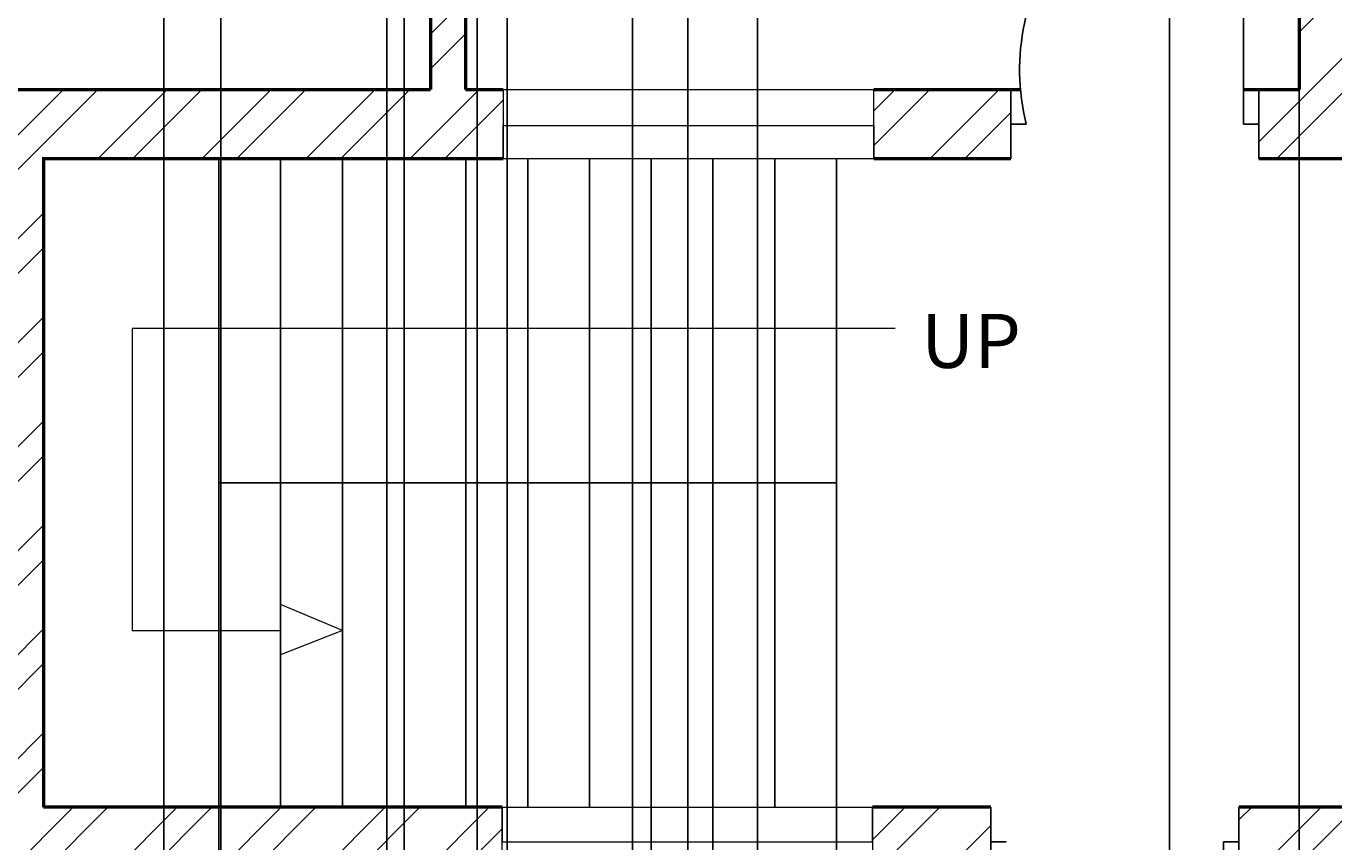
# Model space of a CAD drawing. Units: inches. Extents: x 1980 to 2738, y 1471 to 2568.
# Tile 10 of 22: x 2194 to 2363, y 2007 to 2112. Entities that reach past the tile are written whole.
import ezdxf

# ---------------------------------------------------------------- set-up
doc = ezdxf.new("R2010")
doc.units = ezdxf.units.IN
for name, color, linetype, lineweight in [('A-ANNO-DIMS', 2, 'Continuous', 18), ('A-ANNO-SYMB', 60, 'Continuous', 18), ('A-ANNO-TEXT', 7, 'Continuous', 18), ('A-DOOR', 31, 'Continuous', 25), ('A-FLOR-STRS', 60, 'Continuous', 25), ('A-GLAZ', 141, 'Continuous', 18), ('A-WALL', 7, 'Continuous', 50)]:
    doc.layers.add(name, color=color, linetype=linetype, lineweight=lineweight)
doc.layers.add('A-WALL-PATT', color=9, linetype='Continuous', lineweight=13, true_color=0xd19cc7)
doc.styles.get("Standard").update_dxf_attribs({"font": 'arial.ttf'})
doc.dimstyles.get("Standard").update_dxf_attribs({"dimtxt": 0.18, "dimasz": 0.18, "dimexe": 0.18, "dimexo": 0.0625, "dimgap": 0.09, "dimtad": 0, "dimtih": 1, "dimtoh": 1, "dimdec": 4, "dimzin": 0, "dimdsep": 46, "dimtxsty": 'Standard', "dimcen": 0.09, "dimadec": 0, "dimazin": 0, "dimtfac": 1, "dimtdec": 4, "dimtofl": 0, "dimtmove": 0, "dimatfit": 3, "dimfxl": 1, "dimtolj": 1, "dimtzin": 0, "dimarcsym": 0})

# ---------------------------------------------------------------- blocks, each defined once
blk = doc.blocks.new('WIN-48IN-WALL')
for p, q in [((0, 4.5), (0, 9)), ((0, 9), (0, 0)), ((48, 9), (0, 9)), ((48, 0), (48, 9)), ((48, 9), (48, 4.5)), ((48, 4.5), (0, 4.5)), ((0, 0), (48, 0))]:
    blk.add_line(p, q)
blk = doc.blocks.new('*D40')
at = {"layer": 'A-ANNO-DIMS', "color": 0, "lineweight": -2, "transparency": 16777216}
for p, q in [((2218.65, 2053.14), (2218.65, 1533.71)), ((2298.65, 2053.14), (2298.65, 1533.71)), ((2218.83, 1533.89), (2258.43, 1533.89)), ((2298.47, 1533.89), (2258.87, 1533.89))]:
    blk.add_line(p, q, dxfattribs=at)
at = {"layer": 'A-ANNO-DIMS', "color": 0, "transparency": 16777216}
for points in [[(2218.83, 1533.92), (2218.83, 1533.86), (2218.65, 1533.89)], [(2298.47, 1533.92), (2298.47, 1533.86), (2298.65, 1533.89)]]:
    blk.add_solid(points, dxfattribs=at)
at = {"layer": 'Defpoints', "color": 0, "transparency": 16777216}
for p in [(2218.65, 2053.21), (2298.65, 2053.21), (2298.65, 1533.89)]:
    blk.add_point(p, dxfattribs=at)
at = {"layer": 'A-ANNO-DIMS', "color": 0, "transparency": 16777216, "insert": (2258.65, 1533.89), "char_height": 0.18, "attachment_point": 5}
blk.add_mtext('\\A1;80', dxfattribs=at)
blk = doc.blocks.new('*D41')
at = {"layer": 'A-ANNO-DIMS', "color": 0, "lineweight": -2, "transparency": 16777216}
for p, q in [((2298.65, 2095.14), (2298.65, 1533.71)), ((2515.4, 2095.14), (2515.4, 1533.71)), ((2298.83, 1533.89), (2406.56, 1533.89)), ((2515.22, 1533.89), (2407.49, 1533.89))]:
    blk.add_line(p, q, dxfattribs=at)
at = {"layer": 'A-ANNO-DIMS', "color": 0, "transparency": 16777216}
for points in [[(2298.83, 1533.92), (2298.83, 1533.86), (2298.65, 1533.89)], [(2515.22, 1533.92), (2515.22, 1533.86), (2515.4, 1533.89)]]:
    blk.add_solid(points, dxfattribs=at)
at = {"layer": 'Defpoints', "color": 0, "transparency": 16777216}
for p in [(2298.65, 2095.21), (2515.4, 2095.21), (2515.4, 1533.89)]:
    blk.add_point(p, dxfattribs=at)
at = {"layer": 'A-ANNO-DIMS', "color": 0, "transparency": 16777216, "insert": (2407.03, 1533.89), "char_height": 0.18, "attachment_point": 5}
blk.add_mtext('\\A1;216.75', dxfattribs=at)
blk = doc.blocks.new('*D44')
at = {"layer": 'A-ANNO-DIMS', "color": 0, "lineweight": -2, "transparency": 16777216}
for p, q in [((2218.88, 1694.77), (2218.88, 2507.54)), ((2219.06, 2507.36), (2229.18, 2507.36)), ((2240.22, 2507.36), (2230.11, 2507.36)), ((2240.4, 1694.77), (2240.4, 2507.54))]:
    blk.add_line(p, q, dxfattribs=at)
at = {"layer": 'A-ANNO-DIMS', "color": 0, "transparency": 16777216}
for points in [[(2219.06, 2507.39), (2219.06, 2507.33), (2218.88, 2507.36)], [(2240.22, 2507.39), (2240.22, 2507.33), (2240.4, 2507.36)]]:
    blk.add_solid(points, dxfattribs=at)
at = {"layer": 'Defpoints', "color": 0, "transparency": 16777216}
for p in [(2240.4, 2507.36), (2218.88, 1694.71), (2240.4, 1694.71)]:
    blk.add_point(p, dxfattribs=at)
at = {"layer": 'A-ANNO-DIMS', "color": 0, "transparency": 16777216, "insert": (2229.64, 2507.36), "char_height": 0.18, "attachment_point": 5}
blk.add_mtext('\\A1;21.525', dxfattribs=at)
blk = doc.blocks.new('*D45')
at = {"layer": 'A-ANNO-DIMS', "color": 0, "lineweight": -2, "transparency": 16777216}
for p, q in [((2255.99, 1694.77), (2255.99, 2507.54)), ((2256.17, 2507.36), (2267.22, 2507.36)), ((2279.21, 2507.36), (2268.15, 2507.36)), ((2279.39, 1694.77), (2279.39, 2507.54))]:
    blk.add_line(p, q, dxfattribs=at)
at = {"layer": 'A-ANNO-DIMS', "color": 0, "transparency": 16777216}
for points in [[(2256.17, 2507.39), (2256.17, 2507.33), (2255.99, 2507.36)], [(2279.21, 2507.39), (2279.21, 2507.33), (2279.39, 2507.36)]]:
    blk.add_solid(points, dxfattribs=at)
at = {"layer": 'Defpoints', "color": 0, "transparency": 16777216}
for p in [(2279.39, 2507.36), (2255.99, 1694.71), (2279.39, 1694.71)]:
    blk.add_point(p, dxfattribs=at)
at = {"layer": 'A-ANNO-DIMS', "color": 0, "transparency": 16777216, "insert": (2267.69, 2507.36), "char_height": 0.18, "attachment_point": 5}
blk.add_mtext('\\A1;23.407', dxfattribs=at)
blk = doc.blocks.new('*D46')
at = {"layer": 'A-ANNO-DIMS', "color": 0, "lineweight": -2, "transparency": 16777216}
for p, q in [((2211.52, 1814.77), (2211.52, 2507.54)), ((2211.7, 2507.36), (2226.69, 2507.36)), ((2242.46, 2507.36), (2227.48, 2507.36)), ((2242.64, 1814.77), (2242.64, 2507.54))]:
    blk.add_line(p, q, dxfattribs=at)
at = {"layer": 'A-ANNO-DIMS', "color": 0, "transparency": 16777216}
for points in [[(2211.7, 2507.39), (2211.7, 2507.33), (2211.52, 2507.36)], [(2242.46, 2507.39), (2242.46, 2507.33), (2242.64, 2507.36)]]:
    blk.add_solid(points, dxfattribs=at)
at = {"layer": 'Defpoints', "color": 0, "transparency": 16777216}
for p in [(2242.64, 2507.36), (2211.52, 1814.71), (2242.64, 1814.71)]:
    blk.add_point(p, dxfattribs=at)
at = {"layer": 'A-ANNO-DIMS', "color": 0, "transparency": 16777216, "insert": (2227.08, 2507.36), "char_height": 0.18, "attachment_point": 5}
blk.add_mtext('\\A1;31.12', dxfattribs=at)
blk = doc.blocks.new('*D50')
at = {"layer": 'A-ANNO-DIMS', "color": 0, "lineweight": -2, "transparency": 16777216}
for p, q in [((2288.43, 1708.09), (2288.43, 2507.54)), ((2288.61, 2507.36), (2314.71, 2507.36)), ((2341.6, 2507.36), (2315.5, 2507.36)), ((2341.78, 1708.09), (2341.78, 2507.54))]:
    blk.add_line(p, q, dxfattribs=at)
at = {"layer": 'A-ANNO-DIMS', "color": 0, "transparency": 16777216}
for points in [[(2288.61, 2507.39), (2288.61, 2507.33), (2288.43, 2507.36)], [(2341.6, 2507.39), (2341.6, 2507.33), (2341.78, 2507.36)]]:
    blk.add_solid(points, dxfattribs=at)
at = {"layer": 'Defpoints', "color": 0, "transparency": 16777216}
for p in [(2341.78, 2507.36), (2288.43, 1708.03), (2341.78, 1708.03)]:
    blk.add_point(p, dxfattribs=at)
at = {"layer": 'A-ANNO-DIMS', "color": 0, "transparency": 16777216, "insert": (2315.11, 2507.36), "char_height": 0.18, "attachment_point": 5}
blk.add_mtext('\\A1;53.34', dxfattribs=at)
blk = doc.blocks.new('*D51')
at = {"layer": 'A-ANNO-DIMS', "color": 0, "lineweight": -2, "transparency": 16777216}
for p, q in [((2341.78, 1708.09), (2341.78, 2507.54)), ((2341.96, 2507.36), (2349.72, 2507.36)), ((2358.4, 2507.36), (2350.63, 2507.36)), ((2358.58, 1694.77), (2358.58, 2507.54))]:
    blk.add_line(p, q, dxfattribs=at)
at = {"layer": 'A-ANNO-DIMS', "color": 0, "transparency": 16777216}
for points in [[(2341.96, 2507.39), (2341.96, 2507.33), (2341.78, 2507.36)], [(2358.4, 2507.39), (2358.4, 2507.33), (2358.58, 2507.36)]]:
    blk.add_solid(points, dxfattribs=at)
at = {"layer": 'Defpoints', "color": 0, "transparency": 16777216}
for p in [(2358.58, 2507.36), (2341.78, 1708.03), (2358.58, 1694.71)]:
    blk.add_point(p, dxfattribs=at)
at = {"layer": 'A-ANNO-DIMS', "color": 0, "transparency": 16777216, "insert": (2350.18, 2507.36), "char_height": 0.18, "attachment_point": 5}
blk.add_mtext('\\A1;16.807', dxfattribs=at)
blk = doc.blocks.new('*D54')
at = {"layer": 'A-ANNO-DIMS', "color": 0, "lineweight": -2, "transparency": 16777216}
for p, q in [((2252.1, 1949.01), (2252.1, 2507.54)), ((2252.28, 2507.36), (2261.78, 2507.36)), ((2272.03, 2507.36), (2262.53, 2507.36)), ((2272.21, 1949.01), (2272.21, 2507.54))]:
    blk.add_line(p, q, dxfattribs=at)
at = {"layer": 'A-ANNO-DIMS', "color": 0, "transparency": 16777216}
for points in [[(2252.28, 2507.39), (2252.28, 2507.33), (2252.1, 2507.36)], [(2272.03, 2507.39), (2272.03, 2507.33), (2272.21, 2507.36)]]:
    blk.add_solid(points, dxfattribs=at)
at = {"layer": 'Defpoints', "color": 0, "transparency": 16777216}
for p in [(2272.21, 2507.36), (2252.1, 1948.95), (2272.21, 1948.95)]:
    blk.add_point(p, dxfattribs=at)
at = {"layer": 'A-ANNO-DIMS', "color": 0, "transparency": 16777216, "insert": (2262.16, 2507.36), "char_height": 0.18, "attachment_point": 5}
blk.add_mtext('\\A1;20.11', dxfattribs=at)
blk = doc.blocks.new('*D66')
at = {"layer": 'A-ANNO-DIMS', "color": 0, "lineweight": -2, "transparency": 16777216}
for p, q in [((2274.65, 2095.14), (2274.65, 1533.71)), ((2282.65, 2095.14), (2282.65, 1533.71)), ((2274.83, 1533.89), (2278.5, 1533.89)), ((2282.47, 1533.89), (2278.8, 1533.89))]:
    blk.add_line(p, q, dxfattribs=at)
at = {"layer": 'A-ANNO-DIMS', "color": 0, "transparency": 16777216}
for points in [[(2274.83, 1533.92), (2274.83, 1533.86), (2274.65, 1533.89)], [(2282.47, 1533.92), (2282.47, 1533.86), (2282.65, 1533.89)]]:
    blk.add_solid(points, dxfattribs=at)
at = {"layer": 'Defpoints', "color": 0, "transparency": 16777216}
for p in [(2274.65, 2095.21), (2282.65, 2095.21), (2282.65, 1533.89)]:
    blk.add_point(p, dxfattribs=at)
at = {"layer": 'A-ANNO-DIMS', "color": 0, "transparency": 16777216, "insert": (2278.65, 1533.89), "char_height": 0.18, "attachment_point": 5}
blk.add_mtext('\\A1;8', dxfattribs=at)

msp = doc.modelspace()

# ---------------------------------------------------------------- hatches: boundary and pattern name
at = {"layer": 'A-WALL-PATT'}
h = msp.add_hatch(dxfattribs=at)
h.set_pattern_fill('ANSI32', color=256)
h.paths.add_polyline_path([(2257.5661, 2416.2064), (2257.5661, 2420.7064), (2250.5833, 2420.7064), (2250.5833, 2462.7064), (2246.0833, 2462.7064), (2246.0833, 2420.7064), (2237.0791, 2420.7064), (2237.0791, 2411.7064), (2246.0833, 2411.7064), (2246.0833, 2291.7064), (2242.6109, 2291.7064), (2242.6109, 2287.2064), (2246.0833, 2287.2064), (2250.5833, 2287.2064), (2250.5833, 2291.7064), (2250.5833, 2411.7064), (2257.5661, 2411.7064)])
h.paths.add_polyline_path([(2387.0396, 2416.2064), (2387.0396, 2420.7064), (2367.5833, 2420.7064), (2367.5833, 2462.7064), (2358.5833, 2462.7064), (2358.5833, 2420.7064), (2329.3087, 2420.7064), (2329.3087, 2411.7064), (2358.5833, 2411.7064), (2358.5833, 2321.7275), (2358.5833, 2309.7064), (2347.3089, 2309.7064), (2293.3089, 2309.7064), (2293.3089, 2259.0771), (2297.8089, 2259.0771), (2297.8089, 2305.2064), (2347.3089, 2305.2064), (2347.3089, 2284.7412), (2351.8089, 2284.7412), (2351.8089, 2305.2064), (2372.3188, 2305.2064), (2372.3761, 2284.3899), (2377.0295, 2284.3899), (2377.0295, 2299.3058), (2377.0295, 2305.2064), (2426.5295, 2305.2064), (2426.5295, 2257.5573), (2431.0295, 2257.5573), (2431.0295, 2309.7064), (2377.0295, 2309.7064), (2367.5833, 2309.7064), (2367.5833, 2321.7275), (2367.5833, 2411.7064), (2387.0396, 2411.7064)])
h.paths.add_polyline_path([(2448.5267, 2416.2064), (2448.5267, 2420.7064), (2423.0396, 2420.7064), (2423.0396, 2411.7064), (2448.5267, 2411.7064)])
h.paths.add_polyline_path([(2130.9128, 2416.2064), (2130.9128, 2420.7064), (2105.0833, 2420.7064), (2105.0833, 2386.6942), (2114.0833, 2386.6942), (2114.0833, 2411.7064), (2130.9128, 2411.7064)])
h.paths.add_polyline_path([(2212.9478, 2420.7064), (2190.9128, 2420.7064), (2190.9128, 2411.7064), (2212.9478, 2411.7064), (2212.9478, 2416.2064)])
h.paths.add_polyline_path([(2114.0833, 2326.6942), (2105.0833, 2326.6942), (2105.0833, 2291.7064), (2081.0833, 2291.7064), (2081.0833, 2287.2064), (2105.0833, 2287.2064), (2105.0833, 2276.1935), (2114.0833, 2276.1935), (2114.0833, 2287.2064), (2166.3825, 2287.2064), (2166.3825, 2289.4564), (2166.3825, 2291.7064), (2114.0833, 2291.7064)])
h.paths.add_polyline_path([(2114.0833, 2252.1935), (2105.0833, 2252.1935), (2105.0833, 2233.2064), (2081.0833, 2233.2064), (2081.0833, 2228.7064), (2105.0833, 2228.7064), (2105.0833, 2213.4478), (2114.0833, 2213.4478), (2114.0833, 2228.7064), (2195.0833, 2228.7064), (2199.5833, 2228.7064), (2208.4455, 2228.7064), (2208.4455, 2230.9564), (2208.4455, 2233.2064), (2199.5833, 2233.2064), (2199.5833, 2287.2064), (2206.8904, 2287.2064), (2206.8904, 2289.4564), (2206.8904, 2291.7064), (2189.446, 2291.7064), (2189.446, 2289.4564), (2189.446, 2287.2064), (2195.0833, 2287.2064), (2195.0833, 2233.2064), (2114.0833, 2233.2064)])
h.paths.add_polyline_path([(2114.0833, 2153.4478), (2109.5833, 2153.4478), (2105.0833, 2153.4478), (2105.0833, 2135.2374), (2114.0833, 2135.2374)], flags=17)
h.paths.add_polyline_path([(2135.9619, 2095.4081), (2140.1805, 2095.4081), (2140.1805, 2104.2064), (2114.0833, 2104.2064), (2114.0833, 2110.3997), (2109.5833, 2110.3997), (2105.0833, 2110.3997), (2105.0833, 2104.2064), (2081.0833, 2104.2064), (2081.0833, 2099.7064), (2105.0833, 2099.7064), (2127.5416, 2099.8532), (2127.5416, 2056.9393), (2136.2133, 2056.9393)], flags=17)
h.paths.add_polyline_path([(2255.4895, 2104.2064), (2250.5833, 2104.2064), (2250.5833, 2233.2064), (2246.0833, 2233.2064), (2242.4941, 2233.2064), (2242.4941, 2228.7064), (2246.0833, 2228.7064), (2246.0833, 2104.2064), (2163.6825, 2104.2064), (2163.6825, 2099.8072), (2163.6825, 2095.4081), (2191.4325, 2095.4081), (2191.4325, 2011.2064), (2186.0833, 2011.2064), (2136.5143, 2010.8824), (2136.3702, 2032.9403), (2131.9559, 2032.9115), (2127.5416, 2032.8826), (2127.5416, 2006.7064), (2105.0833, 2006.7064), (2081.0833, 2006.7064), (2081.0833, 2002.2064), (2105.0833, 2002.2064), (2105.0833, 1995.9329), (2114.0833, 1995.9329), (2114.0833, 2002.2064), (2246.0833, 2002.2064), (2246.0833, 1877.7064), (2242.1358, 1877.7064), (2242.1358, 1873.2064), (2250.5833, 1873.2064), (2250.5833, 2002.2064), (2255.3335, 2002.2064), (2255.3335, 2011.2064), (2195.9325, 2011.2064), (2195.9325, 2095.2064), (2255.4895, 2095.2064), (2255.4895, 2099.5471)])
h.paths.add_polyline_path([(2199.5833, 1873.2064), (2209.827, 1873.2064), (2209.827, 1875.4564), (2209.827, 1877.7064), (2114.0833, 1877.7064), (2114.0833, 1890.0968), (2105.0833, 1890.0968), (2105.0833, 1877.7064), (2081.0833, 1877.7064), (2081.0833, 1873.2064), (2105.0833, 1873.2064), (2105.0833, 1857.7279), (2114.0833, 1857.7279), (2114.0833, 1873.2064), (2195.0833, 1873.2064), (2195.0833, 1819.2064), (2190.298, 1819.2064), (2190.298, 1814.7064), (2209.8976, 1814.7064), (2209.8976, 1816.9564), (2209.8976, 1819.2064), (2199.5833, 1819.2064)])
h.paths.add_polyline_path([(2114.0833, 1814.7064), (2166.2538, 1814.7064), (2166.2538, 1816.9564), (2166.2538, 1819.2064), (2114.0833, 1819.2064), (2114.0833, 1833.7279), (2109.5833, 1833.7279), (2105.0833, 1833.7279), (2105.0833, 1819.2064), (2081.0833, 1819.2064), (2081.0833, 1814.7064), (2105.0833, 1814.7064), (2105.0833, 1782.5516), (2114.0833, 1782.5516)])
h.paths.add_polyline_path([(2114.0833, 1722.5516), (2109.5833, 1722.5516), (2105.0833, 1722.5516), (2105.0833, 1685.7064), (2124.5104, 1685.7064), (2124.5104, 1690.2064), (2124.5104, 1694.7064), (2114.0833, 1694.7064)])
h.paths.add_polyline_path([(2218.8787, 1694.7064), (2184.5104, 1694.7064), (2184.5104, 1685.7064), (2218.8787, 1685.7064), (2218.8787, 1690.2064)])
h.paths.add_polyline_path([(2250.5833, 1819.2064), (2242.6431, 1819.2064), (2242.6431, 1816.9564), (2242.6431, 1814.7064), (2246.0833, 1814.7064), (2246.0833, 1694.7064), (2240.4035, 1694.7064), (2240.4035, 1690.2064), (2240.4035, 1685.7064), (2246.0833, 1685.7064), (2246.0833, 1643.7064), (2250.5833, 1643.7064), (2250.5833, 1685.7064), (2255.9859, 1685.7064), (2255.9859, 1690.2064), (2255.9859, 1694.7064), (2250.5833, 1694.7064)])
h.paths.add_polyline_path([(2297.4764, 1694.7064), (2279.3934, 1694.7064), (2279.3934, 1690.2064), (2279.3934, 1685.7064), (2297.4764, 1685.7064), (2297.4764, 1690.2064)])
h.paths.add_polyline_path([(2377.1596, 1694.7064), (2367.5833, 1694.7064), (2367.5833, 1787.7064), (2431.0295, 1787.7064), (2431.0295, 1792.2064), (2431.0295, 1849.4149), (2428.7795, 1849.4149), (2426.5295, 1849.4149), (2426.5295, 1792.2064), (2421.5833, 1792.2064), (2367.5833, 1792.2064), (2297.8089, 1792.2064), (2297.8089, 1850.2946), (2295.5589, 1850.2946), (2293.3089, 1850.2946), (2293.3089, 1792.2064), (2293.3089, 1787.7064), (2297.8089, 1787.7064), (2358.5833, 1787.7064), (2358.5833, 1694.7064), (2333.4764, 1694.7064), (2333.4764, 1685.7064), (2358.5833, 1685.7064), (2358.5833, 1643.7064), (2367.5833, 1643.7064), (2367.5833, 1685.7064), (2377.1596, 1685.7064)])
h.paths.add_polyline_path([(2442.4912, 1694.7064), (2413.1596, 1694.7064), (2413.1596, 1685.7064), (2442.4912, 1685.7064)])
h.paths.add_polyline_path([(2480.0833, 1814.7064), (2483.4816, 1814.7064), (2483.4816, 1817.9384), (2483.4816, 1819.2064), (2475.5833, 1819.2064), (2475.5833, 1694.7064), (2470.7283, 1694.7064), (2470.7283, 1685.7064), (2475.5833, 1685.7064), (2475.5833, 1643.7064), (2480.0833, 1643.7064), (2480.0833, 1685.7064), (2486.3293, 1685.7064), (2486.3293, 1690.2064), (2486.3293, 1694.7064), (2480.0833, 1694.7064)])
h.paths.add_polyline_path([(2621.0833, 1721.7349), (2612.0833, 1721.7349), (2612.0833, 1694.7064), (2586.1453, 1694.7064), (2586.1453, 1685.7064), (2621.0833, 1685.7064)])
h.paths.add_polyline_path([(2526.1453, 1690.2064), (2526.1453, 1694.7064), (2511.584, 1694.7064), (2511.584, 1690.2064), (2511.584, 1685.7064), (2526.1453, 1685.7064)])
h.paths.add_polyline_path([(2645.0833, 1819.2064), (2621.0833, 1819.2064), (2621.0833, 1835.8527), (2616.5833, 1835.8527), (2612.0833, 1835.8527), (2612.0833, 1819.2064), (2560.2541, 1819.2064), (2560.2541, 1814.7064), (2612.0833, 1814.7064), (2612.0833, 1781.7349), (2621.0833, 1781.7349), (2621.0833, 1814.7064), (2645.0833, 1814.7064)])
h.paths.add_polyline_path([(2645.0833, 1877.7064), (2621.0833, 1877.7064), (2621.0833, 1886.4375), (2612.0833, 1886.4375), (2612.0833, 1877.7064), (2517.1032, 1877.7064), (2517.1032, 1875.4564), (2517.1032, 1873.2064), (2526.5833, 1873.2064), (2526.5833, 1819.2064), (2516.6454, 1819.2064), (2516.6454, 1816.9564), (2516.6454, 1814.7064), (2536.4445, 1814.7064), (2536.4445, 1816.9564), (2536.4445, 1819.2064), (2531.0833, 1819.2064), (2531.0833, 1873.2064), (2612.0833, 1873.2064), (2612.0833, 1859.8527), (2621.0833, 1859.8527), (2621.0833, 1873.2064), (2645.0833, 1873.2064)])
h.paths.add_polyline_path([(2645.0833, 2006.7064), (2621.0833, 2006.7064), (2588.5085, 2006.7064), (2588.5085, 2052.9125), (2579.9045, 2052.9125), (2579.9045, 2011.2064), (2519.9045, 2011.2064), (2519.9045, 2095.2064), (2553.1204, 2095.2064), (2553.1204, 2104.2064), (2480.0833, 2104.2064), (2480.0833, 2228.7064), (2484.3832, 2228.7064), (2484.3832, 2230.9564), (2484.3832, 2233.2064), (2475.5833, 2233.2064), (2475.5833, 2104.2064), (2463.1308, 2104.2064), (2463.1308, 2095.2064), (2501.2463, 2095.2064), (2510.9045, 2095.2064), (2515.4045, 2095.2064), (2515.4045, 2011.2064), (2510.9045, 2011.2064), (2501.2463, 2011.2064), (2462.5957, 2011.2064), (2462.5957, 2002.2064), (2475.5833, 2002.2064), (2475.5833, 1873.2064), (2483.6146, 1873.2064), (2483.6146, 1875.4564), (2483.6146, 1877.7064), (2480.0833, 1877.7064), (2480.0833, 2002.2064), (2612.0833, 2002.2064), (2612.0833, 1996.309), (2621.0833, 1996.309), (2621.0833, 2002.2064), (2645.0833, 2002.2064)])
h.paths.add_polyline_path([(2588.5085, 2099.7277), (2621.0833, 2099.7277), (2645.0833, 2099.7064), (2645.0833, 2104.2064), (2621.0833, 2104.2064), (2621.0833, 2109.0038), (2616.5833, 2109.0038), (2612.0833, 2109.0038), (2612.0833, 2104.2064), (2575.0621, 2104.2064), (2575.0621, 2099.7064), (2575.0621, 2095.2064), (2579.9045, 2095.2064), (2579.9045, 2076.9125), (2588.5085, 2076.9125)], flags=17)
h.paths.add_polyline_path([(2367.5833, 2002.2064), (2373.7228, 2002.2064), (2373.7228, 2006.7064), (2373.7228, 2011.2064), (2350.7889, 2011.2064), (2350.7889, 2006.7064), (2350.7889, 2002.2064), (2358.5833, 2002.2064), (2358.5833, 1877.7064), (2293.3089, 1877.7064), (2293.3089, 1870.4987), (2297.8089, 1870.4987), (2297.8089, 1873.2064), (2347.3089, 1873.2064), (2347.3089, 1847.2208), (2351.8089, 1847.2208), (2351.8089, 1873.2064), (2372.5295, 1873.2064), (2372.5295, 1847.8619), (2377.0295, 1847.8619), (2377.0295, 1873.2064), (2426.5295, 1873.2064), (2426.5295, 1868.7339), (2431.0295, 1868.7339), (2431.0295, 1877.7064), (2367.5833, 1877.7064)])
h.paths.add_polyline_path([(2531.0833, 2287.2064), (2534.2285, 2287.2064), (2534.2285, 2291.7064), (2516.7886, 2291.7064), (2516.7886, 2287.2064), (2526.5833, 2287.2064), (2526.5833, 2233.2064), (2517.9112, 2233.2064), (2517.9112, 2230.9564), (2517.9112, 2228.7064), (2526.5833, 2228.7064), (2531.0833, 2228.7064), (2612.0833, 2228.7064), (2612.0833, 2206.8504), (2621.0833, 2206.8504), (2621.0833, 2228.7064), (2645.0833, 2228.7064), (2645.0833, 2233.2064), (2621.0833, 2233.2064), (2621.0833, 2241.8536), (2616.5833, 2241.8536), (2612.0833, 2241.8536), (2612.0833, 2233.2064), (2531.0833, 2233.2064)])
h.paths.add_polyline_path([(2645.0833, 2291.7064), (2621.0833, 2291.7064), (2621.0833, 2323.0138), (2616.5833, 2323.0138), (2612.0833, 2323.0138), (2612.0833, 2291.7064), (2559.6852, 2291.7064), (2559.6852, 2289.4564), (2559.6852, 2287.2064), (2612.0833, 2287.2064), (2612.0833, 2265.8536), (2621.0833, 2265.8536), (2621.0833, 2287.2064), (2645.0833, 2287.2064)])
h.paths.add_polyline_path([(2621.0833, 2420.7064), (2582.8189, 2420.7064), (2582.8189, 2411.7064), (2612.0833, 2411.7064), (2612.0833, 2383.0138), (2621.0833, 2383.0138)])
h.paths.add_polyline_path([(2480.0833, 2411.7064), (2485.7342, 2411.7064), (2485.7342, 2416.2064), (2485.7342, 2420.7064), (2480.0833, 2420.7064), (2480.0833, 2462.7064), (2475.5833, 2462.7064), (2475.5833, 2420.7064), (2469.4083, 2420.7064), (2469.4083, 2411.7064), (2475.5833, 2411.7064), (2475.5833, 2291.7064), (2475.5833, 2287.2064), (2482.9195, 2287.2064), (2482.9195, 2289.4564), (2482.9195, 2291.7064), (2480.0833, 2291.7064)])
h.paths.add_polyline_path([(2367.5833, 2228.7064), (2431.0295, 2228.7064), (2431.0295, 2233.2064), (2431.0295, 2237.4203), (2428.7795, 2237.4203), (2426.5295, 2237.4203), (2426.5295, 2233.2064), (2377.0295, 2233.2064), (2377.0295, 2260.3837), (2372.4423, 2260.3837), (2372.517, 2233.2635), (2351.8089, 2233.2064), (2351.8089, 2260.7412), (2347.3089, 2260.7412), (2347.3089, 2233.2064), (2297.8089, 2233.2064), (2297.8089, 2236.9324), (2293.3089, 2236.9324), (2293.3089, 2228.7064), (2358.5833, 2228.7064), (2358.5833, 2104.2064), (2353.3665, 2104.2064), (2353.3665, 2095.2064), (2373.8869, 2095.2064), (2373.8869, 2099.7064), (2373.8869, 2104.2064), (2367.5833, 2104.2064)])
h.paths.add_polyline_path([(2321.2323, 2104.2064), (2303.4895, 2104.2064), (2303.4895, 2095.2064), (2321.2323, 2095.2064), (2321.2323, 2099.7064)], flags=0)
h.paths.add_polyline_path([(2415.1308, 2099.7064), (2415.1308, 2104.2064), (2404.81, 2104.2064), (2404.81, 2095.2064), (2415.1308, 2095.2064)], flags=17)
h.paths.add_polyline_path([(2318.6336, 2011.2064), (2303.3335, 2011.2064), (2303.3335, 2002.2064), (2318.6336, 2002.2064)], flags=0)
h.paths.add_polyline_path([(2414.5957, 2011.2064), (2406.2461, 2011.2064), (2406.2461, 2006.7064), (2406.2461, 2002.2064), (2414.5957, 2002.2064)], flags=17)
h = msp.add_hatch(dxfattribs=at)
h.set_pattern_fill('ANSI32', color=256)
h.paths.add_polyline_path([(2321.2323, 2104.2064), (2303.4895, 2104.2064), (2303.4895, 2095.2064), (2321.2323, 2095.2064), (2321.2323, 2099.7064)])
h.paths.add_polyline_path([(2318.6336, 2011.2064), (2303.3335, 2011.2064), (2303.3335, 2002.2064), (2318.6336, 2002.2064)])
h.paths.add_polyline_path([(2114.0833, 1972.9983), (2109.5833, 1972.9983), (2105.0833, 1972.9983), (2105.0833, 1950.0968), (2114.0833, 1950.0968)])
h.paths.add_polyline_path([(2621.0833, 1971.9446), (2616.5833, 1971.9446), (2612.0833, 1971.9446), (2612.0833, 1946.4375), (2621.0833, 1946.4375)])
h.paths.add_polyline_path([(2621.0833, 2146.8504), (2612.0833, 2146.8504), (2612.0833, 2134.6713), (2621.0833, 2134.6713)])

# ---------------------------------------------------------------- linework, layer by layer
at = {"layer": 'A-ANNO-SYMB'}
for p, q in [((2306.2358, 2073.2192), (2207.4154, 2073.2192)), ((2207.4154, 2073.2192), (2207.4154, 2034.0737)), ((2234.6516, 2034.0737), (2226.6516, 2037.4799)), ((2226.6516, 2037.4799), (2226.6516, 2031.723)), ((2207.4154, 2034.0737), (2226.6516, 2034.0737)), ((2234.6516, 2034.0737), (2226.6516, 2030.9342))]:
    msp.add_line(p, q, dxfattribs=at)
at = {"layer": 'A-DOOR'}
for p, q in [((2351.3665, 2099.7064), (2351.3665, 2123.7064)), ((2321.2323, 2104.2064), (2321.2323, 2095.2064)), ((2353.3665, 2104.2064), (2353.3665, 2095.2064)), ((2321.2323, 2095.2064), (2321.2323, 2099.7064)), ((2321.2323, 2099.7064), (2321.2323, 2099.7064)), ((2321.2323, 2099.7064), (2323.2323, 2099.7064)), ((2353.3665, 2099.7064), (2351.3665, 2099.7064)), ((2353.3665, 2095.2064), (2353.3665, 2099.7064)), ((2318.6336, 2002.2064), (2318.6336, 2011.2064)), ((2318.6336, 2011.2064), (2318.6336, 2006.7064)), ((2350.7889, 2002.2064), (2350.7889, 2011.2064)), ((2350.7889, 2011.2064), (2350.7889, 2006.7064)), ((2318.6336, 2006.7064), (2320.6336, 2006.7064)), ((2350.7889, 2006.7064), (2348.7889, 2006.7064)), ((2348.7889, 2006.7064), (2348.7889, 1970.7064))]:
    msp.add_line(p, q, dxfattribs=at)
msp.add_arc((2351.3665, 2106.7129), 28.9935, 90, 193.984358, dxfattribs=at)
at = {"layer": 'A-FLOR-STRS'}
for p, q in [((2218.6516, 2095.2064), (2218.6516, 2011.2064)), ((2226.6516, 2095.2064), (2226.6516, 2011.2064)), ((2234.6516, 2095.2064), (2234.6516, 2011.2064)), ((2242.6516, 2095.2064), (2242.6516, 2011.2064)), ((2250.6516, 2095.2064), (2250.6516, 2011.2064)), ((2258.6516, 2095.2064), (2258.6516, 2011.2064)), ((2266.6516, 2095.2064), (2266.6516, 2011.2064)), ((2274.6516, 2095.2064), (2274.6516, 2011.2064)), ((2282.6516, 2095.2064), (2282.6516, 2011.2064)), ((2290.6516, 2095.2064), (2290.6516, 2011.2064)), ((2298.6516, 2095.2064), (2298.6516, 2011.2064)), ((2218.6516, 2053.2064), (2298.6516, 2053.2064))]:
    msp.add_line(p, q, dxfattribs=at)
at = {"layer": 'A-GLAZ'}
for p, q in [((2255.4895, 2104.2064), (2255.4895, 2095.2064)), ((2255.4895, 2104.2064), (2303.4895, 2104.2064)), ((2303.4895, 2095.2064), (2303.4895, 2104.2064)), ((2255.4895, 2095.2064), (2255.4895, 2099.5471)), ((2255.4895, 2099.5471), (2303.4895, 2099.5471)), ((2303.4895, 2099.5471), (2303.4895, 2095.2064)), ((2303.4895, 2095.2064), (2255.4895, 2095.2064))]:
    msp.add_line(p, q, dxfattribs=at)
at = {"layer": 'A-WALL'}
for p, q in [((2250.5833, 2233.2064), (2250.5833, 2104.2064)), ((2246.0833, 2228.7064), (2246.0833, 2104.2064)), ((2358.5833, 2228.7064), (2358.5833, 2104.2064)), ((2163.6825, 2104.2064), (2246.0833, 2104.2064)), ((2250.5833, 2104.2064), (2255.4895, 2104.2064)), ((2303.4895, 2104.2064), (2322.4815, 2104.2064)), ((2351.3665, 2104.2064), (2358.5833, 2104.2064)), ((2195.9325, 2095.4081), (2195.9325, 2011.2064)), ((2255.4895, 2095.2064), (2195.9325, 2095.2064)), ((2321.2323, 2095.2064), (2303.4895, 2095.2064)), ((2373.8869, 2095.2064), (2353.3665, 2095.2064)), ((2246.0833, 2011.2064), (2195.9325, 2011.2064)), ((2195.9325, 2011.2064), (2195.9325, 2011.2064)), ((2255.3335, 2011.2064), (2195.9325, 2011.2064)), ((2318.6336, 2011.2064), (2303.3335, 2011.2064)), ((2373.7228, 2011.2064), (2350.7889, 2011.2064))]:
    msp.add_line(p, q, dxfattribs=at)

# ---------------------------------------------------------------- block references
at = {"layer": 'A-GLAZ', "extrusion": (0, 0, -1), "zscale": -1}
msp.add_blockref('WIN-48IN-WALL', (-2303.3339, 2002.206), dxfattribs=at)

# ---------------------------------------------------------------- texts
at = {"layer": 'A-ANNO-TEXT', "insert": (2309.6098, 2075.1169), "char_height": 7, "attachment_point": 1}
msp.add_mtext_dynamic_manual_height_columns('UP', width=15.226412, gutter_width=12.5, heights=[0], dxfattribs=at)

# ---------------------------------------------------------------- dimensions: what is measured, and where the dimension line sits
at = {"layer": 'A-ANNO-DIMS'}
for base, p1, p2, override, picture, middle in [((2242.6431, 2507.3564), (2211.5238, 1814.7064), (2242.6431, 1814.7064), {"dimdec": 2, "dimlfac": 1, "dimrnd": 0, "dimzin": 0, "dimdsep": 46, "dimlunit": 2}, '*D46', (2227.0835, 2507.3564)), ((2240.4035, 2507.3564), (2218.8787, 1694.7064), (2240.4035, 1694.7064), {"dimdec": 3, "dimlfac": 1, "dimrnd": 0, "dimzin": 0, "dimdsep": 46, "dimlunit": 2}, '*D44', (2229.6411, 2507.3564)), ((2272.2106, 2507.3564), (2252.1, 1948.9472), (2272.2106, 1948.9472), {"dimdec": 2, "dimlfac": 1, "dimrnd": 0, "dimzin": 0, "dimdsep": 46, "dimlunit": 2}, '*D54', (2262.1553, 2507.3564)), ((2279.39337, 2507.35642), (2255.98588, 1694.70642), (2279.39337, 1694.70642), {"dimdec": 3, "dimlfac": 1, "dimrnd": 0, "dimzin": 0, "dimdsep": 46, "dimlunit": 2}, '*D45', (2267.68962, 2507.35642)), ((2341.776, 2507.3564), (2288.4349, 1708.0291), (2341.776, 1708.0291), {"dimdec": 2, "dimlfac": 1, "dimrnd": 0, "dimzin": 0, "dimdsep": 46, "dimlunit": 2}, '*D50', (2315.1054, 2507.3564)), ((2358.5833, 2507.3564), (2341.776, 1708.0291), (2358.5833, 1694.7064), {"dimdec": 3, "dimlfac": 1, "dimrnd": 0, "dimzin": 0, "dimdsep": 46, "dimlunit": 2}, '*D51', (2350.1796, 2507.3564)), ((2282.6516, 1533.8857), (2274.6516, 2095.2064), (2282.6516, 2095.2064), {"dimdec": 0, "dimlfac": 1, "dimrnd": 0, "dimzin": 0, "dimdsep": 46, "dimlunit": 2}, '*D66', (2278.6516, 1533.8857)), ((2515.4045, 1533.8857), (2298.6516, 2095.2064), (2515.4045, 2095.2064), {"dimdec": 2, "dimlfac": 1, "dimrnd": 0, "dimzin": 0, "dimdsep": 46, "dimlunit": 2}, '*D41', (2407.0281, 1533.8857)), ((2298.6516, 1533.8857), (2218.6516, 2053.2064), (2298.6516, 2053.2064), {"dimdec": 0, "dimlfac": 1, "dimrnd": 0, "dimzin": 0, "dimdsep": 46, "dimlunit": 2}, '*D40', (2258.6516, 1533.8857))]:
    dim = msp.add_linear_dim(base=base, p1=p1, p2=p2, dimstyle='Standard', override=override, dxfattribs=at)
    dim.commit()
    dim.dimension.update_dxf_attribs({"geometry": picture, "text_midpoint": middle})

doc.saveas('drawing.dxf')
